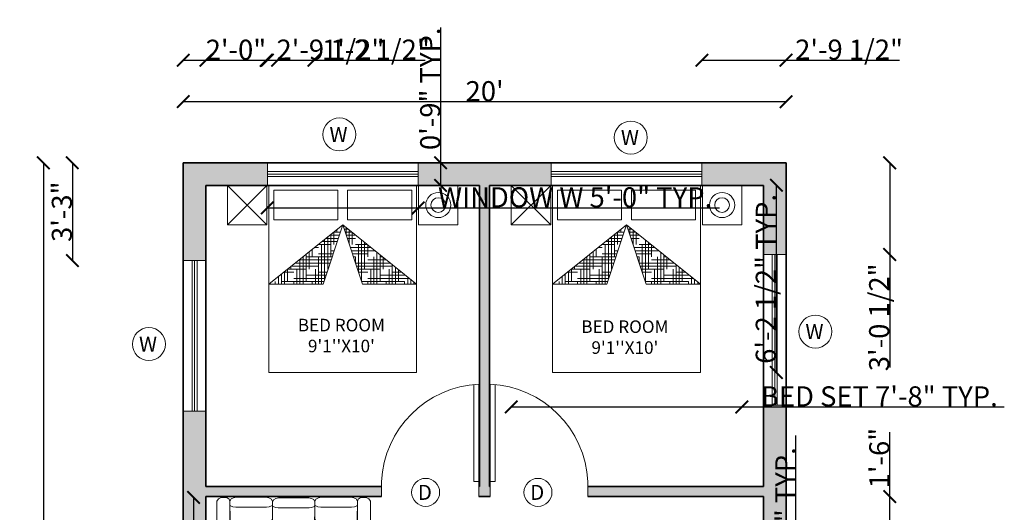
# Model space of a CAD drawing. Units: inches. Extents: x 2163 to 2555, y 1763 to 2232.
# Tile 3 of 3: x 2163 to 2555, y 2035 to 2232. Entities that reach past the tile are written whole.
import ezdxf

# ---------------------------------------------------------------- set-up
doc = ezdxf.new("R2010")
doc.units = ezdxf.units.IN
for name, color, linetype, lineweight in [('A-ANNO-DIMS', 2, 'Continuous', 18), ('A-ANNO-SYMB', 7, 'Continuous', 18), ('A-AREA-IDEN', 7, 'Continuous', 18), ('A-FURN', 8, 'Continuous', 18), ('A-WALL-PATT', 8, 'Continuous', 13), ('Doors', 222, 'Continuous', 18), ('Walls', 7, 'Continuous', 35), ('Windows', 150, 'Continuous', 18)]:
    doc.layers.add(name, color=color, linetype=linetype, lineweight=lineweight)
doc.styles.get("Standard").update_dxf_attribs({"font": 'arial.ttf'})
doc.dimstyles.get("Standard").update_dxf_attribs({"dimtxt": 8, "dimasz": 5, "dimexe": 0.18, "dimexo": 0.0625, "dimgap": 0.09, "dimtad": 1, "dimdec": 1, "dimzin": 0, "dimdsep": 46, "dimlunit": 4, "dimtxsty": 'Standard', "dimblk": 'ARCHTICK', "dimcen": 0.09, "dimse1": 1, "dimse2": 1, "dimadec": 0, "dimazin": 0, "dimtfac": 1, "dimtdec": 1, "dimtofl": 0, "dimtmove": 0, "dimatfit": 3, "dimfxl": 1, "dimtolj": 1, "dimtzin": 0, "dimarcsym": 0})

# ---------------------------------------------------------------- blocks, each defined once
blk = doc.blocks.new('AP0B05')
for p, q in [((35, 100), (35, 880)), ((75, 100), (75, 878.9)), ((35, 100), (35, -20)), ((815, 100), (815, -20))]:
    blk.add_line(p, q)
blk.add_lwpolyline([(35, 100), (75, 100)])
blk.add_arc((-2.4, 62.6), 818.3, 2.62122, 87.37878)
blk = doc.blocks.new('*X4')
at = {"color": 0}
for p, q in [((20.25, 14.8125), (20.2772, 14.8125)), ((20.1487, 14.7188), (20.2772, 14.7188)), ((20.1562, 14.625), (20.1562, 14.7281)), ((20.1739, 14.75), (20.2772, 14.75)), ((20.1875, 14.75), (20.1875, 14.7669)), ((20.199, 14.7812), (20.2772, 14.7812)), ((20.25, 14.3194), (20.25, 14.75)), ((20.0625, 14.2573), (20.0625, 14.6116)), ((20.0938, 14.375), (20.0938, 14.6504)), ((20.0984, 14.6562), (20.125, 14.6562)), ((20.1236, 14.6875), (20.25, 14.6875)), ((20.125, 14.5), (20.125, 14.6893)), ((20.125, 14.5938), (20.2772, 14.5938)), ((20.2188, 14.3091), (20.2188, 14.625)), ((20.25, 14.625), (20.2772, 14.625)), ((19.9727, 14.5), (20.25, 14.5)), ((19.9979, 14.5312), (20.2772, 14.5312)), ((20, 14.2366), (20, 14.5)), ((20.023, 14.5625), (20.2772, 14.5625)), ((20.0312, 14.2469), (20.0312, 14.5727)), ((20.1875, 14.2987), (20.1875, 14.5)), ((19.9062, 14.375), (19.9062, 14.4174)), ((19.9225, 14.4375), (20, 14.4375)), ((19.9476, 14.4688), (20.125, 14.4688)), ((20.125, 14.4062), (20.2772, 14.4062)), ((20.25, 14.4375), (20.2772, 14.4375)), ((19.8125, 14.1744), (19.8125, 14.3008)), ((19.8219, 14.3125), (20.2291, 14.3125)), ((19.8438, 14.1848), (19.8438, 14.3397)), ((19.875, 14.25), (19.875, 14.3785)), ((19.875, 14.3438), (20.2772, 14.3438)), ((19.9688, 14.2262), (19.9688, 14.375)), ((20, 14.375), (20.2772, 14.375)), ((20.1562, 14.2884), (20.1562, 14.375)), ((19.7465, 14.2188), (19.875, 14.2188)), ((19.75, 14.1537), (19.75, 14.2231)), ((19.7716, 14.25), (20, 14.25)), ((19.7812, 14.1641), (19.7812, 14.262)), ((19.7967, 14.2812), (20.125, 14.2812)), ((19.9375, 14.2159), (19.9375, 14.25)), ((19.7018, 14.0938), (19.7786, 14.0938)), ((19.7188, 14.0726), (19.7188, 14.1136)), ((19.7213, 14.1875), (19.75, 14.1875)), ((19.75, 14.0338), (19.75, 14.1032)), ((19.7812, 13.9949), (19.7812, 14.0929)), ((19.7269, 14.0625), (19.8728, 14.0625)), ((19.752, 14.0312), (19.875, 14.0312)), ((19.8125, 14), (19.8125, 14.0825)), ((19.875, 13.8784), (19.875, 14)), ((19.9062, 13.8396), (19.9062, 14.0514)), ((19.9375, 13.8007), (19.9375, 14.0411)), ((19.9688, 13.875), (19.9688, 14.0307)), ((20, 14), (20, 14.0204)), ((20, 14), (20.0614, 14)), ((20.0625, 13.6454), (20.0625, 13.9996)), ((19.8275, 13.9375), (20.25, 13.9375)), ((19.8526, 13.9062), (20.125, 13.9062)), ((19.875, 13.9688), (20.1557, 13.9688)), ((20.0938, 13.625), (20.0938, 13.9893)), ((20.125, 13.75), (20.125, 13.9789)), ((20.1562, 13.875), (20.1562, 13.9686)), ((20.25, 13.5), (20.25, 13.9375)), ((19.8777, 13.875), (20, 13.875)), ((20, 13.8125), (20.2772, 13.8125)), ((20.0312, 13.6842), (20.0312, 13.875)), ((20.125, 13.8438), (20.2772, 13.8438)), ((20.2188, 13.4511), (20.2188, 13.875)), ((20.25, 13.875), (20.2772, 13.875)), ((19.9532, 13.7812), (20.2772, 13.7812)), ((19.9783, 13.75), (20.25, 13.75)), ((20, 13.723), (20, 13.75)), ((20.0035, 13.7188), (20.125, 13.7188)), ((20.1875, 13.49), (20.1875, 13.75)), ((20.0789, 13.625), (20.2772, 13.625)), ((20.104, 13.5938), (20.2772, 13.5938)), ((20.125, 13.6562), (20.2772, 13.6562)), ((20.1562, 13.5288), (20.1562, 13.625)), ((20.25, 13.6875), (20.2772, 13.6875)), ((20.1292, 13.5625), (20.25, 13.5625)), ((20.25, 13.5), (20.2772, 13.5)), ((20.2046, 13.4688), (20.2772, 13.4688)), ((20.2297, 13.4375), (20.2772, 13.4375)), ((20.2549, 13.4062), (20.2772, 13.4062))]:
    blk.add_line(p, q, dxfattribs=at)
blk = doc.blocks.new('MAT-P13')
for p, q in [((-1.17, 0), (-1.17, -0.4)), ((-1.17, 0), (-0.77, 0)), ((-1.17, -0.4), (-0.77, 0)), ((-0.77, -0.4), (-1.17, 0)), ((-0.77, 0), (-0.77, -0.4)), ((-0.75, 0), (0.75, 0)), ((-0.75, 0), (-0.75, -1.9)), ((0.75, 0), (0.75, -1.9)), ((0.77, 0), (1.17, 0)), ((0.77, 0), (0.77, -0.4)), ((1.17, 0), (1.17, -0.4)), ((-0.7, -0.05), (-0.7, -0.35)), ((-0.7, -0.05), (-0.05, -0.05)), ((-0.05, -0.35), (-0.05, -0.05)), ((0.05, -0.05), (0.7, -0.05)), ((0.05, -0.35), (0.05, -0.05)), ((0.7, -0.05), (0.7, -0.35)), ((-0.7, -0.35), (-0.05, -0.35)), ((0.05, -0.35), (0.7, -0.35)), ((-1.17, -0.4), (-0.77, -0.4)), ((-0.75, -1.0034), (0, -0.4)), ((0, -0.4), (-0.75, -1.0034)), ((0, -0.4), (-0.2, -1.0034)), ((0, -0.4), (0.2, -1.0034)), ((0, -0.4), (0.75, -1.0034)), ((0.77, -0.4), (1.17, -0.4)), ((-0.75, -1.0034), (-0.2, -1.0034)), ((0.2, -1.0034), (0.75, -1.0034)), ((0.75, -1.9), (-0.75, -1.9))]:
    blk.add_line(p, q)
for radius in [0.1279, 0.0749]:
    blk.add_circle((0.97, -0.2), radius)
at = {"xscale": -1, "rotation": 90}
blk.add_blockref('*X4', (14.1285, 19.2738), dxfattribs=at)
blk = doc.blocks.new('12PCOU17')
at = {"color": 0, "linetype": 'ByBlock'}
for points in [[(-34.71, 34.72), (-33.66, 34.31), (-3.27, 34.3), (-1.81, 34.76), (-1.05, 35.2), (-0.38, 36.65), (-0.61, 39.84), (-1.73, 40.94), (-3.27, 41.4), (-33.66, 41.4), (-34.95, 40.5), (-35.65, 39.02), (-35.49, 35.83), (-34.71, 34.72)], [(-1.89, 11.91), (-1.66, 11.91), (-0.35, 14.68), (-0.35, 31.05), (-0.74, 32.58), (-1.89, 33.83), (-33.63, 34.3), (-34.84, 33.63), (-35.43, 32.38), (-35.68, 31), (-35.68, 14.74), (-35.43, 13.36), (-34.66, 11.99), (-33.44, 11.43), (-3, 11.44), (-1.66, 11.91)], [(-31.25, 11.43), (-31.06, 11.84), (-30.6, 13.09), (-30.4, 14.62), (-30.4, 31.12), (-30.6, 32.65), (-31.06, 33.9), (-31.81, 34.3)], [(-23.84, 11.43), (-22.99, 11.9), (-22.46, 13.15), (-22.23, 14.67), (-22.23, 31.07), (-22.46, 32.59), (-22.99, 33.84), (-23.12, 34.3)], [(-1.54, -10.96), (-1.31, -10.96), (0, -8.19), (0, 8.19), (-0.39, 9.71), (-1.54, 10.96), (-33.28, 11.44), (-34.5, 10.77), (-35.08, 9.51), (-35.33, 8.14), (-35.33, -8.13), (-35.08, -9.51), (-34.31, -10.87), (-33.1, -11.44), (-2.65, -11.43), (-1.31, -10.96)], [(-30.9, -11.44), (-30.72, -11.02), (-30.25, -9.77), (-30.05, -8.25), (-30.05, 8.26), (-30.25, 9.78), (-30.72, 11.03), (-31.47, 11.44)], [(-23.49, -11.44), (-22.64, -10.96), (-22.11, -9.72), (-21.88, -8.19), (-21.88, 8.2), (-22.11, 9.73), (-22.64, 10.97), (-22.77, 11.44)], [(-1.89, -11.91), (-1.66, -11.91), (-0.35, -14.68), (-0.35, -31.05), (-0.74, -32.58), (-1.89, -33.83), (-33.63, -34.3), (-34.84, -33.63), (-35.43, -32.38), (-35.68, -31), (-35.68, -14.74), (-35.43, -13.36), (-34.66, -11.99), (-33.44, -11.43), (-3, -11.44), (-1.66, -11.91)], [(-31.25, -11.43), (-31.06, -11.84), (-30.6, -13.09), (-30.4, -14.62), (-30.4, -31.12), (-30.6, -32.65), (-31.06, -33.9), (-31.81, -34.3)], [(-23.84, -11.43), (-22.99, -11.9), (-22.46, -13.15), (-22.23, -14.67), (-22.23, -31.07), (-22.46, -32.59), (-22.99, -33.84), (-23.12, -34.3)], [(-34.71, -34.72), (-33.66, -34.31), (-3.27, -34.3), (-1.81, -34.76), (-1.05, -35.2), (-0.38, -36.65), (-0.61, -39.84), (-1.73, -40.94), (-3.27, -41.4), (-33.66, -41.4), (-34.95, -40.5), (-35.65, -39.02), (-35.49, -35.83), (-34.71, -34.72)]]:
    blk.add_lwpolyline(points, dxfattribs=at)
blk = doc.blocks.new('_ArchTick')
at = {"color": 0, "linetype": 'ByBlock', "const_width": 0.15}
blk.add_lwpolyline([(-0.5, -0.5), (0.5, 0.5)], dxfattribs=at)
blk = doc.blocks.new('*D11')
at = {"layer": 'A-ANNO-DIMS', "color": 0, "lineweight": -2, "transparency": 16777216}
blk.add_line((2228.01, 2198.85), (2468.01, 2198.85), dxfattribs=at)
at = {"layer": 'Defpoints', "color": 0, "transparency": 16777216}
for p in [(2468.01, 2198.85), (2228.01, 2174.5), (2468.01, 2174.5)]:
    blk.add_point(p, dxfattribs=at)
at = {"layer": 'A-ANNO-DIMS', "color": 0, "lineweight": -2, "transparency": 16777216, "xscale": 5, "yscale": 5, "zscale": 5, "rotation": 180}
blk.add_blockref('_ArchTick', (2228.01, 2198.85), dxfattribs=at)
at = {"layer": 'A-ANNO-DIMS', "color": 0, "lineweight": -2, "transparency": 16777216, "xscale": 5, "yscale": 5, "zscale": 5}
blk.add_blockref('_ArchTick', (2468.01, 2198.85), dxfattribs=at)
at = {"layer": 'A-ANNO-DIMS', "color": 0, "transparency": 16777216, "insert": (2348.01, 2203.02), "char_height": 8, "attachment_point": 5}
blk.add_mtext("\\A1;20'", dxfattribs=at)
blk = doc.blocks.new('*D12')
at = {"layer": 'A-ANNO-DIMS', "color": 0, "lineweight": -2, "transparency": 16777216}
blk.add_line((2172.33, 2174.5), (2172.33, 1814.5), dxfattribs=at)
at = {"layer": 'Defpoints', "color": 0, "transparency": 16777216}
for p in [(2228.01, 2174.5), (2172.33, 1814.5), (2228.01, 1814.5)]:
    blk.add_point(p, dxfattribs=at)
at = {"layer": 'A-ANNO-DIMS', "color": 0, "lineweight": -2, "transparency": 16777216, "xscale": 5, "yscale": 5, "zscale": 5}
for p, rotation in [((2172.33, 2174.5), 90), ((2172.33, 1814.5), 270)]:
    blk.add_blockref('_ArchTick', p, dxfattribs=dict(at, rotation=rotation))
at = {"layer": 'A-ANNO-DIMS', "color": 0, "transparency": 16777216, "insert": (2168.15, 1994.5), "char_height": 8, "attachment_point": 5, "rotation": 90}
blk.add_mtext("\\A1;30'", dxfattribs=at)
blk = doc.blocks.new('WIN-60IN')
for p, q in [((0, 5.5), (60, 5.5)), ((0, 4.5), (60, 4.5)), ((0, 3.5), (60, 3.5))]:
    blk.add_line(p, q)
blk.add_lwpolyline([(0, 9), (60, 9), (60, 0), (0, 0)], close=True)
blk = doc.blocks.new('TAG-WINDOW-W')
blk.add_circle((6.57, 6.57), 6.57)
blk.add_text('W', height=6).set_placement((2.61, 3.57))
blk = doc.blocks.new('TAG-DOOR-D')
blk.add_circle((5.58, 5.58), 5.58)
blk.add_text('D', height=6).set_placement((2.46, 2.58))
blk = doc.blocks.new('*D18')
at = {"layer": 'A-ANNO-DIMS', "color": 0, "lineweight": -2, "transparency": 16777216}
for p, q in [((2261.51, 2156.5), (2321.51, 2156.5)), ((2321.51, 2156.5), (2441.58, 2156.5))]:
    blk.add_line(p, q, dxfattribs=at)
at = {"layer": 'Defpoints', "color": 0, "transparency": 16777216}
for p in [(2261.51, 2165.5), (2321.51, 2165.5), (2321.51, 2156.5)]:
    blk.add_point(p, dxfattribs=at)
at = {"layer": 'A-ANNO-DIMS', "color": 0, "lineweight": -2, "transparency": 16777216, "xscale": 5, "yscale": 5, "zscale": 5, "rotation": 180}
blk.add_blockref('_ArchTick', (2261.51, 2156.5), dxfattribs=at)
at = {"layer": 'A-ANNO-DIMS', "color": 0, "lineweight": -2, "transparency": 16777216, "xscale": 5, "yscale": 5, "zscale": 5}
blk.add_blockref('_ArchTick', (2321.51, 2156.5), dxfattribs=at)
at = {"layer": 'A-ANNO-DIMS', "color": 0, "transparency": 16777216, "insert": (2384.04, 2160.73), "char_height": 8, "attachment_point": 5}
blk.add_mtext('\\A1;WINDOW W 5\'-0" TYP.', dxfattribs=at)
blk = doc.blocks.new('*D19')
at = {"layer": 'A-ANNO-DIMS', "color": 0, "lineweight": -2, "transparency": 16777216}
for p, q in [((2330.51, 2174.5), (2330.51, 2228.45)), ((2330.51, 2165.5), (2330.51, 2174.5))]:
    blk.add_line(p, q, dxfattribs=at)
at = {"layer": 'Defpoints', "color": 0, "transparency": 16777216}
for p in [(2321.51, 2174.5), (2330.51, 2174.5), (2321.51, 2165.5)]:
    blk.add_point(p, dxfattribs=at)
at = {"layer": 'A-ANNO-DIMS', "color": 0, "lineweight": -2, "transparency": 16777216, "xscale": 5, "yscale": 5, "zscale": 5}
for p, rotation in [((2330.51, 2174.5), 90), ((2330.51, 2165.5), 270)]:
    blk.add_blockref('_ArchTick', p, dxfattribs=dict(at, rotation=rotation))
at = {"layer": 'A-ANNO-DIMS', "color": 0, "transparency": 16777216, "insert": (2326.34, 2203.98), "char_height": 8, "attachment_point": 5, "rotation": 90}
blk.add_mtext('\\A1;0\'-9" TYP.', dxfattribs=at)
blk = doc.blocks.new('*D26')
at = {"layer": 'A-ANNO-DIMS', "color": 0, "lineweight": -2, "transparency": 16777216}
for p, q in [((2358.62, 2077.21), (2450.4, 2077.21)), ((2450.4, 2077.21), (2554.92, 2077.21))]:
    blk.add_line(p, q, dxfattribs=at)
at = {"layer": 'Defpoints', "color": 0, "transparency": 16777216}
for p in [(2358.62, 2090.97), (2450.4, 2090.97), (2450.4, 2077.21)]:
    blk.add_point(p, dxfattribs=at)
at = {"layer": 'A-ANNO-DIMS', "color": 0, "lineweight": -2, "transparency": 16777216, "xscale": 5, "yscale": 5, "zscale": 5, "rotation": 180}
blk.add_blockref('_ArchTick', (2358.62, 2077.21), dxfattribs=at)
at = {"layer": 'A-ANNO-DIMS', "color": 0, "lineweight": -2, "transparency": 16777216, "xscale": 5, "yscale": 5, "zscale": 5}
blk.add_blockref('_ArchTick', (2450.4, 2077.21), dxfattribs=at)
at = {"layer": 'A-ANNO-DIMS', "color": 0, "transparency": 16777216, "insert": (2505.16, 2081.43), "char_height": 8, "attachment_point": 5}
blk.add_mtext('\\A1;BED SET 7\'-8" TYP.', dxfattribs=at)
blk = doc.blocks.new('*D27')
at = {"layer": 'A-ANNO-DIMS', "color": 0, "lineweight": -2, "transparency": 16777216}
blk.add_line((2464.17, 2090.97), (2464.17, 2165.5), dxfattribs=at)
at = {"layer": 'Defpoints', "color": 0, "transparency": 16777216}
for p in [(2450.4, 2165.5), (2464.17, 2165.5), (2450.4, 2090.97)]:
    blk.add_point(p, dxfattribs=at)
at = {"layer": 'A-ANNO-DIMS', "color": 0, "lineweight": -2, "transparency": 16777216, "xscale": 5, "yscale": 5, "zscale": 5}
for p, rotation in [((2464.17, 2165.5), 90), ((2464.17, 2090.97), 270)]:
    blk.add_blockref('_ArchTick', p, dxfattribs=dict(at, rotation=rotation))
at = {"layer": 'A-ANNO-DIMS', "color": 0, "transparency": 16777216, "insert": (2459.95, 2128.24), "char_height": 8, "attachment_point": 5, "rotation": 90}
blk.add_mtext('\\A1;6\'-2 1/2" TYP.', dxfattribs=at)
blk = doc.blocks.new('*D28')
at = {"layer": 'A-ANNO-DIMS', "color": 0, "lineweight": -2, "transparency": 16777216}
for p, q in [((2471.96, 1882.16), (2471.96, 2065.78)), ((2471.96, 1855.84), (2471.96, 1882.16))]:
    blk.add_line(p, q, dxfattribs=at)
at = {"layer": 'Defpoints', "color": 0, "transparency": 16777216}
for p in [(2468.01, 1882.16), (2471.96, 1882.16), (2468.01, 1855.84)]:
    blk.add_point(p, dxfattribs=at)
at = {"layer": 'A-ANNO-DIMS', "color": 0, "lineweight": -2, "transparency": 16777216, "xscale": 5, "yscale": 5, "zscale": 5}
for p, rotation in [((2471.96, 1882.16), 90), ((2471.96, 1855.84), 270)]:
    blk.add_blockref('_ArchTick', p, dxfattribs=dict(at, rotation=rotation))
at = {"layer": 'A-ANNO-DIMS', "color": 0, "transparency": 16777216, "insert": (2467.73, 1976.47), "char_height": 8, "attachment_point": 5, "rotation": 90}
blk.add_mtext('\\A1;COMPACT WINDOW 2\'-2 1/2" TYP.', dxfattribs=at)
blk = doc.blocks.new('*D39')
at = {"layer": 'A-ANNO-DIMS', "color": 0, "lineweight": -2, "transparency": 16777216}
for p, q in [((2232.15, 2041.21), (2232.15, 2014.8)), ((2232.15, 2014.8), (2232.15, 1969.58))]:
    blk.add_line(p, q, dxfattribs=at)
at = {"layer": 'Defpoints', "color": 0, "transparency": 16777216}
for p in [(2241.35, 2041.21), (2232.15, 2014.8), (2241.35, 2014.8)]:
    blk.add_point(p, dxfattribs=at)
at = {"layer": 'A-ANNO-DIMS', "color": 0, "lineweight": -2, "transparency": 16777216, "xscale": 5, "yscale": 5, "zscale": 5}
for p, rotation in [((2232.15, 2041.21), 90), ((2232.15, 2014.8), 270)]:
    blk.add_blockref('_ArchTick', p, dxfattribs=dict(at, rotation=rotation))
at = {"layer": 'A-ANNO-DIMS', "color": 0, "transparency": 16777216, "insert": (2227.93, 1989.69), "char_height": 8, "attachment_point": 5, "rotation": 90}
blk.add_mtext('\\A1;2\'-2 1/2"', dxfattribs=at)
blk = doc.blocks.new('*D42')
at = {"layer": 'A-ANNO-DIMS', "color": 0, "lineweight": -2, "transparency": 16777216}
for p, q in [((2228.01, 2215.35), (2261.51, 2215.35)), ((2261.51, 2215.35), (2306.73, 2215.35))]:
    blk.add_line(p, q, dxfattribs=at)
at = {"layer": 'Defpoints', "color": 0, "transparency": 16777216}
for p in [(2261.51, 2215.35), (2228.01, 2174.5), (2261.51, 2174.5)]:
    blk.add_point(p, dxfattribs=at)
at = {"layer": 'A-ANNO-DIMS', "color": 0, "lineweight": -2, "transparency": 16777216, "xscale": 5, "yscale": 5, "zscale": 5, "rotation": 180}
blk.add_blockref('_ArchTick', (2228.01, 2215.35), dxfattribs=at)
at = {"layer": 'A-ANNO-DIMS', "color": 0, "lineweight": -2, "transparency": 16777216, "xscale": 5, "yscale": 5, "zscale": 5}
blk.add_blockref('_ArchTick', (2261.51, 2215.35), dxfattribs=at)
at = {"layer": 'A-ANNO-DIMS', "color": 0, "transparency": 16777216, "insert": (2286.62, 2219.58), "char_height": 8, "attachment_point": 5}
blk.add_mtext('\\A1;2\'-9 1/2"', dxfattribs=at)
blk = doc.blocks.new('*D43')
at = {"layer": 'A-ANNO-DIMS', "color": 0, "lineweight": -2, "transparency": 16777216}
for p, q in [((2434.51, 2215.35), (2468.01, 2215.35)), ((2468.01, 2215.35), (2513.23, 2215.35))]:
    blk.add_line(p, q, dxfattribs=at)
at = {"layer": 'Defpoints', "color": 0, "transparency": 16777216}
for p in [(2468.01, 2215.35), (2434.51, 2174.5), (2468.01, 2174.5)]:
    blk.add_point(p, dxfattribs=at)
at = {"layer": 'A-ANNO-DIMS', "color": 0, "lineweight": -2, "transparency": 16777216, "xscale": 5, "yscale": 5, "zscale": 5, "rotation": 180}
blk.add_blockref('_ArchTick', (2434.51, 2215.35), dxfattribs=at)
at = {"layer": 'A-ANNO-DIMS', "color": 0, "lineweight": -2, "transparency": 16777216, "xscale": 5, "yscale": 5, "zscale": 5}
blk.add_blockref('_ArchTick', (2468.01, 2215.35), dxfattribs=at)
at = {"layer": 'A-ANNO-DIMS', "color": 0, "transparency": 16777216, "insert": (2493.12, 2219.58), "char_height": 8, "attachment_point": 5}
blk.add_mtext('\\A1;2\'-9 1/2"', dxfattribs=at)
blk = doc.blocks.new('*D44')
at = {"layer": 'A-ANNO-DIMS', "color": 0, "lineweight": -2, "transparency": 16777216}
blk.add_line((2183.86, 2174.5), (2183.86, 2135.5), dxfattribs=at)
at = {"layer": 'Defpoints', "color": 0, "transparency": 16777216}
for p in [(2228.01, 2174.5), (2183.86, 2135.5), (2228.01, 2135.5)]:
    blk.add_point(p, dxfattribs=at)
at = {"layer": 'A-ANNO-DIMS', "color": 0, "lineweight": -2, "transparency": 16777216, "xscale": 5, "yscale": 5, "zscale": 5}
for p, rotation in [((2183.86, 2174.5), 90), ((2183.86, 2135.5), 270)]:
    blk.add_blockref('_ArchTick', p, dxfattribs=dict(at, rotation=rotation))
at = {"layer": 'A-ANNO-DIMS', "color": 0, "transparency": 16777216, "insert": (2179.68, 2155), "char_height": 8, "attachment_point": 5, "rotation": 90}
blk.add_mtext('\\A1;3\'-3"', dxfattribs=at)
blk = doc.blocks.new('*D51')
at = {"layer": 'A-ANNO-DIMS', "color": 0, "lineweight": -2, "transparency": 16777216}
for p, q in [((2509.31, 2174.5), (2509.31, 2137.97)), ((2509.31, 2137.97), (2509.31, 2092.89))]:
    blk.add_line(p, q, dxfattribs=at)
at = {"layer": 'Defpoints', "color": 0, "transparency": 16777216}
for p in [(2468.01, 2174.5), (2468.01, 2137.97), (2509.31, 2137.97)]:
    blk.add_point(p, dxfattribs=at)
at = {"layer": 'A-ANNO-DIMS', "color": 0, "lineweight": -2, "transparency": 16777216, "xscale": 5, "yscale": 5, "zscale": 5}
for p, rotation in [((2509.31, 2174.5), 90), ((2509.31, 2137.97), 270)]:
    blk.add_blockref('_ArchTick', p, dxfattribs=dict(at, rotation=rotation))
at = {"layer": 'A-ANNO-DIMS', "color": 0, "transparency": 16777216, "insert": (2505.09, 2112.93), "char_height": 8, "attachment_point": 5, "rotation": 90}
blk.add_mtext('\\A1;3\'-0 1/2"', dxfattribs=at)
blk = doc.blocks.new('*D55')
at = {"layer": 'A-ANNO-DIMS', "color": 0, "lineweight": -2, "transparency": 16777216}
blk.add_line((2237.01, 2215.35), (2261.01, 2215.35), dxfattribs=at)
at = {"layer": 'Defpoints', "color": 0, "transparency": 16777216}
for p in [(2261.01, 2215.35), (2237.01, 1919.5), (2261.01, 1919.5)]:
    blk.add_point(p, dxfattribs=at)
at = {"layer": 'A-ANNO-DIMS', "color": 0, "lineweight": -2, "transparency": 16777216, "xscale": 5, "yscale": 5, "zscale": 5, "rotation": 180}
blk.add_blockref('_ArchTick', (2237.01, 2215.35), dxfattribs=at)
at = {"layer": 'A-ANNO-DIMS', "color": 0, "lineweight": -2, "transparency": 16777216, "xscale": 5, "yscale": 5, "zscale": 5}
blk.add_blockref('_ArchTick', (2261.01, 2215.35), dxfattribs=at)
at = {"layer": 'A-ANNO-DIMS', "color": 0, "transparency": 16777216, "insert": (2249.01, 2219.53), "char_height": 8, "attachment_point": 5}
blk.add_mtext('\\A1;2\'-0"', dxfattribs=at)
blk = doc.blocks.new('*D57')
at = {"layer": 'A-ANNO-DIMS', "color": 0, "lineweight": -2, "transparency": 16777216}
for p, q in [((2509.31, 2041.5), (2509.31, 2067.2)), ((2509.31, 2023.5), (2509.31, 2041.5))]:
    blk.add_line(p, q, dxfattribs=at)
at = {"layer": 'Defpoints', "color": 0, "transparency": 16777216}
for p in [(2459.01, 2041.5), (2509.31, 2041.5), (2459.84, 2023.5)]:
    blk.add_point(p, dxfattribs=at)
at = {"layer": 'A-ANNO-DIMS', "color": 0, "lineweight": -2, "transparency": 16777216, "xscale": 5, "yscale": 5, "zscale": 5}
for p, rotation in [((2509.31, 2041.5), 90), ((2509.31, 2023.5), 270)]:
    blk.add_blockref('_ArchTick', p, dxfattribs=dict(at, rotation=rotation))
at = {"layer": 'A-ANNO-DIMS', "color": 0, "transparency": 16777216, "insert": (2505.14, 2056.85), "char_height": 8, "attachment_point": 5, "rotation": 90}
blk.add_mtext('\\A1;1\'-6"', dxfattribs=at)
blk = doc.blocks.new('*D58')
at = {"layer": 'A-ANNO-DIMS', "color": 0, "lineweight": -2, "transparency": 16777216}
for p, q in [((2265.57, 2215.35), (2280.07, 2215.35)), ((2280.07, 2215.35), (2324.4, 2215.35))]:
    blk.add_line(p, q, dxfattribs=at)
at = {"layer": 'Defpoints', "color": 0, "transparency": 16777216}
for p in [(2280.07, 2215.35), (2265.57, 1844.36), (2280.07, 1844.36)]:
    blk.add_point(p, dxfattribs=at)
at = {"layer": 'A-ANNO-DIMS', "color": 0, "lineweight": -2, "transparency": 16777216, "xscale": 5, "yscale": 5, "zscale": 5, "rotation": 180}
blk.add_blockref('_ArchTick', (2265.57, 2215.35), dxfattribs=at)
at = {"layer": 'A-ANNO-DIMS', "color": 0, "lineweight": -2, "transparency": 16777216, "xscale": 5, "yscale": 5, "zscale": 5}
blk.add_blockref('_ArchTick', (2280.07, 2215.35), dxfattribs=at)
at = {"layer": 'A-ANNO-DIMS', "color": 0, "transparency": 16777216, "insert": (2304.73, 2219.58), "char_height": 8, "attachment_point": 5}
blk.add_mtext('\\A1;1\'-2 1/2"', dxfattribs=at)

msp = doc.modelspace()

# ---------------------------------------------------------------- hatches: boundary and pattern name
at = {"layer": 'A-WALL-PATT', "transparency": 33554585}
h = msp.add_hatch(color=256, dxfattribs=at)
h.dxf.hatch_style = 1
h.paths.add_polyline_path([(2261.51, 2174.5), (2228.01, 2174.5), (2228.01, 2135.5), (2237.01, 2135.5), (2237.01, 2165.5), (2261.51, 2165.5)])
h.paths.add_polyline_path([(2237.01, 2075.5), (2228.01, 2075.5), (2228.01, 2012.5), (2237.01, 2012.5), (2237.01, 2041.5), (2306.96, 2041.5), (2306.96, 2045.5), (2237.01, 2045.5)])
h.paths.add_polyline_path([(2237.01, 1952.5), (2228.01, 1952.5), (2228.01, 1901.5), (2237.01, 1901.5), (2237.01, 1919.5), (2281.23, 1919.5), (2281.23, 1923.5), (2237.01, 1923.5)])
h.paths.add_polyline_path([(2237.01, 1841.5), (2228.01, 1841.5), (2228.01, 1814.5), (2249.01, 1814.5), (2249.01, 1823.5), (2237.01, 1823.5)])
h.paths.add_polyline_path([(2330.01, 1923.5), (2320.02, 1923.5), (2320.02, 1919.5), (2321.01, 1919.5), (2321.01, 1823.5), (2309.01, 1823.5), (2309.01, 1814.5), (2330.01, 1814.5)])
h.paths.add_polyline_path([(2468.01, 1855.84), (2459.01, 1855.84), (2459.01, 1823.5), (2368.01, 1823.5), (2368.01, 1814.5), (2468.01, 1814.5)])
h.paths.add_polyline_path([(2468.01, 1949.34), (2459.01, 1949.34), (2459.01, 1923.5), (2390.01, 1923.5), (2390.01, 2001.5), (2391.3, 2001.5), (2391.3, 2005.5), (2386.01, 2005.5), (2386.01, 1923.5), (2368.01, 1923.5), (2368.01, 1914.5), (2459.01, 1914.5), (2459.01, 1882.16), (2468.01, 1882.16)])
h.paths.add_polyline_path([(2468.01, 2077.97), (2459.01, 2077.97), (2459.01, 2045.5), (2389.06, 2045.5), (2389.06, 2041.5), (2459.01, 2041.5), (2459.01, 2005.5), (2423.94, 2005.5), (2423.94, 2001.5), (2459.01, 2001.5), (2459.01, 1975.66), (2468.01, 1975.66)])
h.paths.add_polyline_path([(2468.01, 2174.5), (2434.51, 2174.5), (2434.51, 2165.5), (2450.4, 2165.5), (2459.01, 2165.5), (2459.01, 2137.97), (2468.01, 2137.97)])
msp.add_hatch(color=256, dxfattribs=at).paths.add_polyline_path([(2374.51, 2174.5), (2321.51, 2174.5), (2321.51, 2165.5), (2321.71, 2165.5), (2337.4, 2165.5), (2346.01, 2165.5), (2346.01, 2045.5), (2345.76, 2041.5), (2350.26, 2041.5), (2350.26, 2045.5), (2350.01, 2045.5), (2350.01, 2165.5), (2374.51, 2165.5)])

# ---------------------------------------------------------------- linework, layer by layer
at = {"layer": 'Walls'}
for p, q in [((2228.01, 2174.5), (2468.01, 2174.5)), ((2228.01, 2174.5), (2228.01, 1814.5)), ((2468.01, 2174.5), (2468.01, 1814.5)), ((2237.01, 2165.5), (2346.01, 2165.5)), ((2237.01, 2165.5), (2237.01, 2045.5)), ((2346.01, 2165.5), (2346.01, 2045.5)), ((2350.01, 2165.5), (2350.01, 2045.5)), ((2350.01, 2165.5), (2459.01, 2165.5)), ((2459.01, 2165.5), (2459.01, 2045.5)), ((2237.01, 2045.5), (2306.96, 2045.5)), ((2345.76, 2045.5), (2346.01, 2045.5)), ((2350.01, 2045.5), (2350.26, 2045.5)), ((2389.06, 2045.5), (2459.01, 2045.5)), ((2237.01, 2041.5), (2306.96, 2041.5)), ((2237.01, 2041.5), (2237.01, 1923.5)), ((2345.76, 2041.5), (2350.26, 2041.5)), ((2389.06, 2041.5), (2459.01, 2041.5)), ((2459.01, 2041.5), (2459.01, 2005.5))]:
    msp.add_line(p, q, dxfattribs=at)

# ---------------------------------------------------------------- block references
at = {"layer": 'A-ANNO-SYMB'}
for name, p in [('TAG-WINDOW-W', (2283.63, 2179.2)), ('TAG-WINDOW-W', (2399.65, 2177.97)), ('TAG-WINDOW-W', (2473.13, 2100.67)), ('TAG-WINDOW-W', (2207.79, 2095.68)), ('TAG-DOOR-D', (2318.94, 2037.6)), ('TAG-DOOR-D', (2363.67, 2037.6))]:
    msp.add_blockref(name, p, dxfattribs=at)
at = {"layer": 'A-FURN', "xscale": 39.22578953606225, "yscale": 39.22578953606225, "zscale": 39.22578953606225}
for p in [(2291.51, 2165.5), (2404.51, 2165.5)]:
    msp.add_blockref('MAT-P13', p, dxfattribs=at)
at = {"layer": 'A-FURN', "xscale": 0.7400239287503789, "yscale": 0.7400239287503789, "zscale": 0.7400239287503789, "rotation": 270}
msp.add_blockref('12PCOU17', (2271.98, 2014.8), dxfattribs=at)
at = {"layer": 'Doors', "yscale": 0.0497371052158267, "zscale": 0.0497371052158267}
for p, xscale in [((2347.5, 2042.5), -0.0497371052158267), ((2348.52, 2042.5), 0.0497371052158267)]:
    msp.add_blockref('AP0B05', p, dxfattribs=dict(at, xscale=xscale))
at = {"layer": 'Windows'}
for p in [(2261.51, 2165.5), (2374.51, 2165.5)]:
    msp.add_blockref('WIN-60IN', p, dxfattribs=at)
for p, rotation in [((2468.01, 2077.97), 89.99999999999935), ((2237.01, 2075.5), 89.9999999999991)]:
    msp.add_blockref('WIN-60IN', p, dxfattribs=dict(at, rotation=rotation))

# ---------------------------------------------------------------- texts
at = {"layer": 'A-AREA-IDEN', "char_height": 5, "attachment_point": 1}
for insert in [(2270.69, 2112.33), (2383.56, 2111.7)]:
    msp.add_mtext_dynamic_manual_height_columns("\\pxqc;BED ROOM\\P9'1''X10'", width=40.594, gutter_width=12.5, heights=[0], dxfattribs=dict(at, insert=insert))

# ---------------------------------------------------------------- dimensions: what is measured, and where the dimension line sits
at = {"layer": 'A-ANNO-DIMS'}
for base, p1, p2, override, picture, middle in [((2261.51, 2215.35), (2228.01, 2174.5), (2261.51, 2174.5), {"dimdec": 1, "dimlfac": 1, "dimrnd": 0, "dimzin": 1, "dimdsep": 46, "dimlunit": 4, "dimfrac": 2}, '*D42', (2286.62, 2219.58)), ((2280.07, 2215.35), (2265.57, 1844.36), (2280.07, 1844.36), {"dimdec": 1, "dimlfac": 1, "dimrnd": 0, "dimzin": 1, "dimdsep": 46, "dimlunit": 4, "dimfrac": 2}, '*D58', (2304.73, 2219.58)), ((2468.01, 2215.35), (2434.51, 2174.5), (2468.01, 2174.5), {"dimdec": 1, "dimlfac": 1, "dimrnd": 0, "dimzin": 1, "dimdsep": 46, "dimlunit": 4, "dimfrac": 2}, '*D43', (2493.12, 2219.58)), ((2261.01, 2215.35), (2237.01, 1919.5), (2261.01, 1919.5), {"dimdec": 1, "dimlfac": 1, "dimrnd": 0, "dimzin": 1, "dimdsep": 46, "dimlunit": 4, "dimfrac": 2}, '*D55', (2249.01, 2219.53)), ((2468.01, 2198.85), (2228.01, 2174.5), (2468.01, 2174.5), {"dimclrd": 0, "dimclre": 0, "dimclrt": 0}, '*D11', (2348.01, 2203.02))]:
    dim = msp.add_linear_dim(base=base, p1=p1, p2=p2, dimstyle='Standard', override=override, dxfattribs=at)
    dim.commit()
    dim.dimension.update_dxf_attribs({"geometry": picture, "text_midpoint": middle})
for base, p1, p2, text, picture, middle in [((2330.51, 2174.5), (2321.51, 2165.5), (2321.51, 2174.5), '<> TYP.', '*D19', (2326.34, 2203.98)), ((2464.17, 2165.5), (2450.4, 2090.97), (2450.4, 2165.5), '<> TYP.', '*D27', (2459.95, 2128.24)), ((2471.96, 1882.16), (2468.01, 1855.84), (2468.01, 1882.16), 'COMPACT WINDOW <> TYP.', '*D28', (2467.73, 1976.47))]:
    dim = msp.add_linear_dim(base=base, p1=p1, p2=p2, angle=90, text=text, dimstyle='Standard', override={"dimdec": 1, "dimlfac": 1, "dimrnd": 0, "dimzin": 1, "dimdsep": 46, "dimlunit": 4, "dimfrac": 2}, dxfattribs=at)
    dim.commit()
    dim.dimension.update_dxf_attribs({"geometry": picture, "text_midpoint": middle})
for base, p1, p2, text, picture, middle in [((2321.51, 2156.5), (2261.51, 2165.5), (2321.51, 2165.5), 'WINDOW W <> TYP.', '*D18', (2384.04, 2160.73)), ((2450.4, 2077.21), (2358.62, 2090.97), (2450.4, 2090.97), 'BED SET <> TYP.', '*D26', (2505.16, 2081.43))]:
    dim = msp.add_linear_dim(base=base, p1=p1, p2=p2, text=text, dimstyle='Standard', override={"dimdec": 1, "dimlfac": 1, "dimrnd": 0, "dimzin": 1, "dimdsep": 46, "dimlunit": 4, "dimfrac": 2}, dxfattribs=at)
    dim.commit()
    dim.dimension.update_dxf_attribs({"geometry": picture, "text_midpoint": middle})
for base, p1, p2, angle, override, picture, middle in [((2172.33, 1814.5), (2228.01, 2174.5), (2228.01, 1814.5), 90, {"dimclrd": 0, "dimclre": 0, "dimclrt": 0}, '*D12', (2168.15, 1994.5)), ((2183.86, 2135.5), (2228.01, 2174.5), (2228.01, 2135.5), 90, {"dimdec": 1, "dimlfac": 1, "dimrnd": 0, "dimzin": 1, "dimdsep": 46, "dimlunit": 4, "dimfrac": 2}, '*D44', (2179.68, 2155)), ((2509.31, 2137.97), (2468.01, 2174.5), (2468.01, 2137.97), 90, {"dimdec": 1, "dimlfac": 1, "dimrnd": 0, "dimzin": 1, "dimdsep": 46, "dimlunit": 4, "dimfrac": 2}, '*D51', (2505.09, 2112.93)), ((2509.31, 2041.5), (2459.84, 2023.5), (2459.01, 2041.5), 90, {"dimdec": 1, "dimlfac": 1, "dimrnd": 0, "dimzin": 1, "dimdsep": 46, "dimlunit": 4, "dimfrac": 2}, '*D57', (2505.14, 2056.85)), ((2232.15, 2014.8), (2241.35, 2041.21), (2241.35, 2014.8), 270, {"dimdec": 1, "dimlfac": 1, "dimrnd": 0, "dimzin": 1, "dimdsep": 46, "dimlunit": 4, "dimfrac": 2}, '*D39', (2227.93, 1989.69))]:
    dim = msp.add_linear_dim(base=base, p1=p1, p2=p2, angle=angle, dimstyle='Standard', override=override, dxfattribs=at)
    dim.commit()
    dim.dimension.update_dxf_attribs({"geometry": picture, "text_midpoint": middle})

doc.saveas('drawing.dxf')
